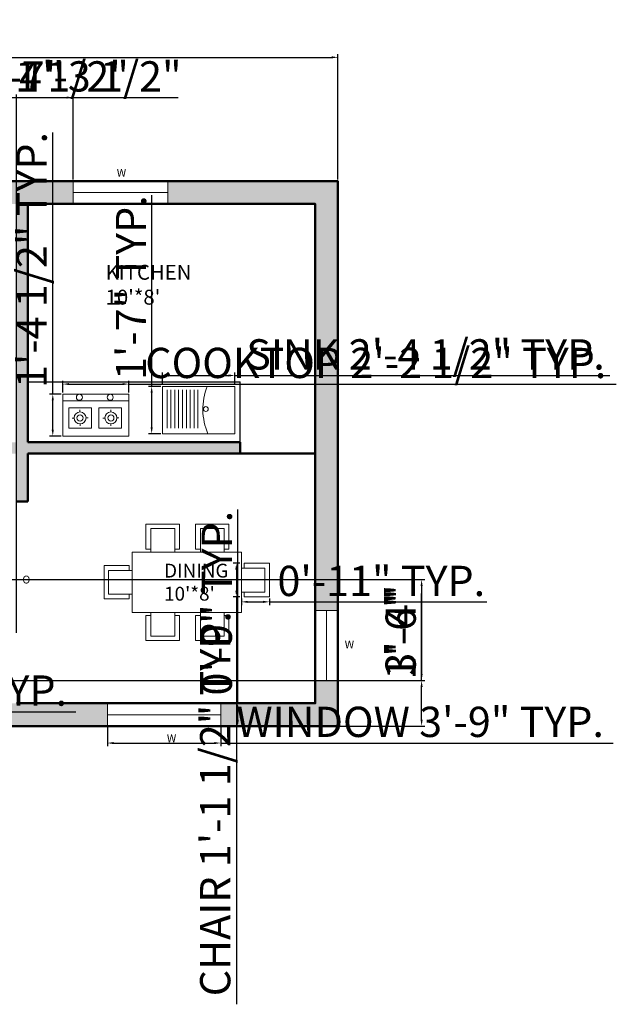
# Model space of a CAD drawing. Units: inches. Extents: x 2225 to 3094, y 1739 to 2599.
# Tile 5 of 5: x 2780 to 3017, y 2108 to 2498. Entities that reach past the tile are written whole.
import ezdxf

# ---------------------------------------------------------------- set-up
doc = ezdxf.new("R2010")
doc.units = ezdxf.units.IN
for name, color, linetype, lineweight in [('A-ANNO-DIMS', 2, 'Continuous', 18), ('A-ANNO-TEXT', 7, 'Continuous', 18), ('A-AREA-IDEN', 7, 'Continuous', 18), ('A-EQPM', 8, 'Continuous', 18), ('A-FLOR-CASE', 9, 'Continuous', 25), ('A-FLOR-FIXT', 9, 'Continuous', 18), ('A-FURN', 8, 'Continuous', 18), ('A-WALL-PATT', 160, 'Continuous', 13), ('WALL', 7, 'Continuous', 50), ('WINDOW', 130, 'Continuous', 18)]:
    doc.layers.add(name, color=color, linetype=linetype, lineweight=lineweight)
doc.styles.get("Standard").update_dxf_attribs({"font": 'arial.ttf'})
doc.dimstyles.new('ISO-25', dxfattribs={"dimtxt": 12, "dimasz": 2.5, "dimexe": 1.25, "dimexo": 0.625, "dimtad": 1, "dimdec": 0, "dimlunit": 4, "dimtxsty": 'Standard', "dimcen": 2.5, "dimadec": 0, "dimazin": 0, "dimtfac": 1, "dimtdec": 0, "dimtmove": 0, "dimatfit": 3, "dimfxl": 1, "dimarcsym": 0})

# ---------------------------------------------------------------- blocks, each defined once
blk = doc.blocks.new('*D5')
at = {"layer": 'A-ANNO-DIMS', "color": 0, "lineweight": -2, "transparency": 16777216}
for p, q in [((2282.56, 2434.95), (2282.56, 2484.67)), ((2285.06, 2483.42), (2904.06, 2483.42)), ((2906.56, 2434.95), (2906.56, 2484.67))]:
    blk.add_line(p, q, dxfattribs=at)
at = {"layer": 'A-ANNO-DIMS', "color": 0, "transparency": 16777216}
for points in [[(2285.06, 2483.83), (2285.06, 2483), (2282.56, 2483.42)], [(2904.06, 2483.83), (2904.06, 2483), (2906.56, 2483.42)]]:
    blk.add_solid(points, dxfattribs=at)
at = {"layer": 'Defpoints', "color": 0, "transparency": 16777216}
for p in [(2906.56, 2483.42), (2282.56, 2434.33), (2906.56, 2434.33)]:
    blk.add_point(p, dxfattribs=at)
at = {"layer": 'A-ANNO-DIMS', "color": 0, "transparency": 16777216, "insert": (2594.56, 2490.17), "char_height": 12, "attachment_point": 5}
blk.add_mtext("52'", dxfattribs=at)
blk = doc.blocks.new('CHAIR-DINING')
for p, q in [((0, 1.13), (0, 11.11)), ((0, 11.11), (13.29, 11.11)), ((13.29, 1.13), (13.29, 11.11)), ((1.95, 1.13), (0, 1.13)), ((13.29, 1.13), (11.43, 1.13))]:
    blk.add_line(p, q)
blk.add_lwpolyline([(1.95, 0), (11.43, 0), (11.43, 9.33), (1.95, 9.33)], close=True)
blk = doc.blocks.new('TABLE-DINING')
blk.add_lwpolyline([(0, 23.93), (43.3, 23.93), (43.3, 0), (0, 0)], close=True)
blk = doc.blocks.new('COOKTOP-TWO-BURNER')
for p, q in [((0, 13.93), (26.27, 13.93)), ((6.81, 9.56), (6.81, 10.38)), ((19.02, 9.56), (19.02, 10.38)), ((4.52, 7.14), (3.73, 7.14)), ((6.9, 4.82), (6.9, 4.11)), ((9.26, 7.23), (10.04, 7.23)), ((16.73, 7.14), (15.94, 7.14)), ((19.11, 4.82), (19.11, 4.11)), ((21.47, 7.23), (22.24, 7.23))]:
    blk.add_line(p, q)
for points in [[(0, 0), (26.27, 0), (26.27, 16.66), (0, 16.66)], [(2.47, 11.19), (11.48, 11.19), (11.48, 3.09), (2.47, 3.09)], [(14.27, 11.19), (23.28, 11.19), (23.28, 3.09), (14.27, 3.09)]]:
    blk.add_lwpolyline(points, close=True)
for centre, radius in [((6.64, 15.37), 1.2), ((18.83, 15.37), 1.2), ((6.89, 7.19), 2.37), ((6.89, 7.19), 1.23), ((19.1, 7.19), 2.37), ((19.1, 7.19), 1.23)]:
    blk.add_circle(centre, radius)
blk = doc.blocks.new('SINK-DRAINBOARD')
for p, q in [((1.79, 17.4), (1.79, 2.15)), ((3.32, 17.4), (3.32, 2.15)), ((4.85, 17.4), (4.85, 2.15)), ((6.38, 17.4), (6.38, 2.15)), ((7.91, 17.4), (7.91, 2.15)), ((9.44, 17.4), (9.44, 2.15)), ((10.98, 17.4), (10.98, 2.15)), ((12.51, 17.4), (12.51, 2.15)), ((14.04, 17.4), (14.04, 2.15))]:
    blk.add_line(p, q)
blk.add_lwpolyline([(0, 0), (28.72, 0), (28.72, 18.77), (0, 18.77)], close=True)
blk.add_circle((17.16, 9.78), 0.951)
blk.add_arc((40.38, 9.7), 24.39, 158.1829, 203.4296)
blk = doc.blocks.new('WIN-37P6IN')
blk.add_line((0, 4.5), (37.6, 4.5))
blk.add_lwpolyline([(37.6, 0), (0, 0), (0, 9), (37.6, 9)], close=True)
blk = doc.blocks.new('WIN-44P9IN')
blk.add_line((0, 4.5), (44.94, 4.5))
blk.add_lwpolyline([(0, 0), (44.94, 0), (44.94, 9), (0, 9)], close=True)
blk = doc.blocks.new('WIN-27P8IN')
blk.add_line((4.5, 0), (4.5, 27.82))
blk.add_lwpolyline([(0, 0), (9, 0), (9, 27.82), (0, 27.82)], close=True)
blk = doc.blocks.new('KITCHEN-COUNTER-RUN')
for p, q in [((0, 0), (0, 24)), ((0, 24), (84.25, 24)), ((84.25, 0), (84.25, 24))]:
    blk.add_line(p, q)
blk = doc.blocks.new('*D28')
at = {"layer": 'A-ANNO-DIMS', "color": 0, "lineweight": -2, "transparency": 16777216}
for p, q in [((2867.63, 2282.83), (2865.01, 2282.83)), ((2866.26, 2280.33), (2866.26, 2272.05)), ((2867.63, 2269.55), (2865.01, 2269.55)), ((2866.26, 2269.55), (2866.26, 2108.01))]:
    blk.add_line(p, q, dxfattribs=at)
at = {"layer": 'A-ANNO-DIMS', "color": 0, "transparency": 16777216}
for points in [[(2865.84, 2280.33), (2866.68, 2280.33), (2866.26, 2282.83)], [(2865.84, 2272.05), (2866.68, 2272.05), (2866.26, 2269.55)]]:
    blk.add_solid(points, dxfattribs=at)
at = {"layer": 'Defpoints', "color": 0, "transparency": 16777216}
for p in [(2868.25, 2282.83), (2866.26, 2269.55), (2868.25, 2269.55)]:
    blk.add_point(p, dxfattribs=at)
at = {"layer": 'A-ANNO-DIMS', "color": 0, "transparency": 16777216, "insert": (2859.43, 2187.53), "char_height": 12, "attachment_point": 5, "rotation": 90}
blk.add_mtext('CHAIR 1\'-1 1/2" TYP.', dxfattribs=at)
blk = doc.blocks.new('*D29')
at = {"layer": 'A-ANNO-DIMS', "color": 0, "lineweight": -2, "transparency": 16777216}
for p, q in [((2868.25, 2268.92), (2868.25, 2266.31)), ((2879.36, 2268.92), (2879.36, 2266.31)), ((2870.75, 2267.56), (2876.86, 2267.56)), ((2879.36, 2267.56), (2965.58, 2267.56))]:
    blk.add_line(p, q, dxfattribs=at)
at = {"layer": 'A-ANNO-DIMS', "color": 0, "transparency": 16777216}
for points in [[(2870.75, 2267.97), (2870.75, 2267.14), (2868.25, 2267.56)], [(2876.86, 2267.97), (2876.86, 2267.14), (2879.36, 2267.56)]]:
    blk.add_solid(points, dxfattribs=at)
at = {"layer": 'Defpoints', "color": 0, "transparency": 16777216}
for p in [(2868.25, 2269.55), (2879.36, 2269.55), (2879.36, 2267.56)]:
    blk.add_point(p, dxfattribs=at)
at = {"layer": 'A-ANNO-DIMS', "color": 0, "transparency": 16777216, "insert": (2923.72, 2274.31), "char_height": 12, "attachment_point": 5}
blk.add_mtext('0\'-11" TYP.', dxfattribs=at)
blk = doc.blocks.new('*D32')
at = {"layer": 'A-ANNO-DIMS', "color": 0, "lineweight": -2, "transparency": 16777216}
for p, q in [((2608.3, 2232.07), (2608.3, 2222.75)), ((2666.2, 2232.07), (2666.2, 2222.75)), ((2610.8, 2224), (2663.7, 2224)), ((2666.2, 2224), (2802.66, 2224))]:
    blk.add_line(p, q, dxfattribs=at)
at = {"layer": 'A-ANNO-DIMS', "color": 0, "transparency": 16777216}
for points in [[(2610.8, 2224.42), (2610.8, 2223.59), (2608.3, 2224)], [(2663.7, 2224.42), (2663.7, 2223.59), (2666.2, 2224)]]:
    blk.add_solid(points, dxfattribs=at)
at = {"layer": 'Defpoints', "color": 0, "transparency": 16777216}
for p in [(2608.3, 2232.69), (2666.2, 2232.69), (2666.2, 2224)]:
    blk.add_point(p, dxfattribs=at)
at = {"layer": 'A-ANNO-DIMS', "color": 0, "transparency": 16777216, "insert": (2735.68, 2230.84), "char_height": 12, "attachment_point": 5}
blk.add_mtext('SOFA 4\'-10" TYP.', dxfattribs=at)
blk = doc.blocks.new('*D38')
at = {"layer": 'A-ANNO-DIMS', "color": 0, "lineweight": -2, "transparency": 16777216}
for p, q in [((2797.42, 2350.57), (2797.42, 2355.14)), ((2799.92, 2353.89), (2821.19, 2353.89)), ((2823.69, 2350.57), (2823.69, 2355.14)), ((2823.69, 2353.89), (3016.9, 2353.89))]:
    blk.add_line(p, q, dxfattribs=at)
at = {"layer": 'A-ANNO-DIMS', "color": 0, "transparency": 16777216}
for points in [[(2799.92, 2354.3), (2799.92, 2353.47), (2797.42, 2353.89)], [(2821.19, 2354.3), (2821.19, 2353.47), (2823.69, 2353.89)]]:
    blk.add_solid(points, dxfattribs=at)
at = {"layer": 'Defpoints', "color": 0, "transparency": 16777216}
for p in [(2823.69, 2353.89), (2797.42, 2349.95), (2823.69, 2349.95)]:
    blk.add_point(p, dxfattribs=at)
at = {"layer": 'A-ANNO-DIMS', "color": 0, "transparency": 16777216, "insert": (2921.55, 2360.72), "char_height": 12, "attachment_point": 5}
blk.add_mtext('COOKTOP 2\'-2 1/2" TYP.', dxfattribs=at)
blk = doc.blocks.new('*D39')
at = {"layer": 'A-ANNO-DIMS', "color": 0, "lineweight": -2, "transparency": 16777216}
for p, q in [((2793.48, 2349.95), (2793.48, 2453.67)), ((2796.79, 2349.95), (2792.23, 2349.95)), ((2793.48, 2335.78), (2793.48, 2347.45)), ((2796.79, 2333.28), (2792.23, 2333.28))]:
    blk.add_line(p, q, dxfattribs=at)
at = {"layer": 'A-ANNO-DIMS', "color": 0, "transparency": 16777216}
for points in [[(2793.06, 2347.45), (2793.89, 2347.45), (2793.48, 2349.95)], [(2793.06, 2335.78), (2793.89, 2335.78), (2793.48, 2333.28)]]:
    blk.add_solid(points, dxfattribs=at)
at = {"layer": 'Defpoints', "color": 0, "transparency": 16777216}
for p in [(2793.48, 2349.95), (2797.42, 2349.95), (2797.42, 2333.28)]:
    blk.add_point(p, dxfattribs=at)
at = {"layer": 'A-ANNO-DIMS', "color": 0, "transparency": 16777216, "insert": (2786.65, 2403.06), "char_height": 12, "attachment_point": 5, "rotation": 90}
blk.add_mtext('1\'-4 1/2" TYP.', dxfattribs=at)
blk = doc.blocks.new('*D40')
at = {"layer": 'A-ANNO-DIMS', "color": 0, "lineweight": -2, "transparency": 16777216}
for p, q in [((2837, 2353.6), (2837, 2358.53)), ((2865.72, 2353.6), (2865.72, 2358.53)), ((2839.5, 2357.28), (2863.22, 2357.28)), ((2865.72, 2357.28), (3014.3, 2357.28))]:
    blk.add_line(p, q, dxfattribs=at)
at = {"layer": 'A-ANNO-DIMS', "color": 0, "transparency": 16777216}
for points in [[(2839.5, 2357.7), (2839.5, 2356.87), (2837, 2357.28)], [(2863.22, 2357.7), (2863.22, 2356.87), (2865.72, 2357.28)]]:
    blk.add_solid(points, dxfattribs=at)
at = {"layer": 'Defpoints', "color": 0, "transparency": 16777216}
for p in [(2865.72, 2357.28), (2837, 2352.98), (2865.72, 2352.98)]:
    blk.add_point(p, dxfattribs=at)
at = {"layer": 'A-ANNO-DIMS', "color": 0, "transparency": 16777216, "insert": (2941.26, 2364.11), "char_height": 12, "attachment_point": 5}
blk.add_mtext('SINK 2\'-4 1/2" TYP.', dxfattribs=at)
blk = doc.blocks.new('*D41')
at = {"layer": 'A-ANNO-DIMS', "color": 0, "lineweight": -2, "transparency": 16777216}
for p, q in [((2832.69, 2352.98), (2832.69, 2428.74)), ((2836.38, 2352.98), (2831.44, 2352.98)), ((2832.69, 2336.71), (2832.69, 2350.48)), ((2836.38, 2334.21), (2831.44, 2334.21))]:
    blk.add_line(p, q, dxfattribs=at)
at = {"layer": 'A-ANNO-DIMS', "color": 0, "transparency": 16777216}
for points in [[(2832.28, 2350.48), (2833.11, 2350.48), (2832.69, 2352.98)], [(2832.28, 2336.71), (2833.11, 2336.71), (2832.69, 2334.21)]]:
    blk.add_solid(points, dxfattribs=at)
at = {"layer": 'Defpoints', "color": 0, "transparency": 16777216}
for p in [(2832.69, 2352.98), (2837, 2352.98), (2837, 2334.21)]:
    blk.add_point(p, dxfattribs=at)
at = {"layer": 'A-ANNO-DIMS', "color": 0, "transparency": 16777216, "insert": (2826.04, 2392.11), "char_height": 12, "attachment_point": 5, "rotation": 90}
blk.add_mtext('1\'-7" TYP.', dxfattribs=at)
blk = doc.blocks.new('*D48')
at = {"layer": 'A-ANNO-DIMS', "color": 0, "lineweight": -2, "transparency": 16777216}
for p, q in [((2815.14, 2217.7), (2815.14, 2210.34)), ((2860.08, 2217.7), (2860.08, 2210.34)), ((2817.64, 2211.59), (2857.58, 2211.59)), ((2860.08, 2211.59), (3015.68, 2211.59))]:
    blk.add_line(p, q, dxfattribs=at)
at = {"layer": 'A-ANNO-DIMS', "color": 0, "transparency": 16777216}
for points in [[(2817.64, 2212), (2817.64, 2211.17), (2815.14, 2211.59)], [(2857.58, 2212), (2857.58, 2211.17), (2860.08, 2211.59)]]:
    blk.add_solid(points, dxfattribs=at)
at = {"layer": 'Defpoints', "color": 0, "transparency": 16777216}
for p in [(2815.14, 2218.33), (2860.08, 2218.33), (2860.08, 2211.59)]:
    blk.add_point(p, dxfattribs=at)
at = {"layer": 'A-ANNO-DIMS', "color": 0, "transparency": 16777216, "insert": (2939.13, 2218.43), "char_height": 12, "attachment_point": 5}
blk.add_mtext('WINDOW 3\'-9" TYP.', dxfattribs=at)
blk = doc.blocks.new('*D49')
at = {"layer": 'A-ANNO-DIMS', "color": 0, "lineweight": -2, "transparency": 16777216}
for p, q in [((2866.82, 2227.33), (2866.82, 2304.22)), ((2860.7, 2227.33), (2868.07, 2227.33)), ((2866.82, 2220.83), (2866.82, 2224.83)), ((2860.7, 2218.33), (2868.07, 2218.33))]:
    blk.add_line(p, q, dxfattribs=at)
at = {"layer": 'A-ANNO-DIMS', "color": 0, "transparency": 16777216}
for points in [[(2866.4, 2224.83), (2867.23, 2224.83), (2866.82, 2227.33)], [(2866.4, 2220.83), (2867.23, 2220.83), (2866.82, 2218.33)]]:
    blk.add_solid(points, dxfattribs=at)
at = {"layer": 'Defpoints', "color": 0, "transparency": 16777216}
for p in [(2860.08, 2227.33), (2866.82, 2227.33), (2860.08, 2218.33)]:
    blk.add_point(p, dxfattribs=at)
at = {"layer": 'A-ANNO-DIMS', "color": 0, "transparency": 16777216, "insert": (2860.06, 2267.03), "char_height": 12, "attachment_point": 5, "rotation": 90}
blk.add_mtext('0\'-9" TYP.', dxfattribs=at)
blk = doc.blocks.new('*D61')
at = {"layer": 'A-ANNO-DIMS', "color": 0, "lineweight": -2, "transparency": 16777216}
for p, q in [((2720.79, 2434.95), (2720.79, 2468.73)), ((2723.29, 2467.48), (2755.89, 2467.48)), ((2758.39, 2434.95), (2758.39, 2468.73)), ((2758.39, 2467.48), (2821.99, 2467.48))]:
    blk.add_line(p, q, dxfattribs=at)
at = {"layer": 'A-ANNO-DIMS', "color": 0, "transparency": 16777216}
for points in [[(2723.29, 2467.89), (2723.29, 2467.06), (2720.79, 2467.48)], [(2755.89, 2467.89), (2755.89, 2467.06), (2758.39, 2467.48)]]:
    blk.add_solid(points, dxfattribs=at)
at = {"layer": 'Defpoints', "color": 0, "transparency": 16777216}
for p in [(2758.39, 2467.48), (2720.79, 2434.33), (2758.39, 2434.33)]:
    blk.add_point(p, dxfattribs=at)
at = {"layer": 'A-ANNO-DIMS', "color": 0, "transparency": 16777216, "insert": (2791.44, 2474.31), "char_height": 12, "attachment_point": 5}
blk.add_mtext('3\'-1 1/2"', dxfattribs=at)
blk = doc.blocks.new('*D62')
at = {"layer": 'A-ANNO-DIMS', "color": 0, "lineweight": -2, "transparency": 16777216}
for p, q in [((2758.39, 2434.95), (2758.39, 2468.73)), ((2760.89, 2467.48), (2799.04, 2467.48)), ((2801.54, 2434.95), (2801.54, 2468.73))]:
    blk.add_line(p, q, dxfattribs=at)
at = {"layer": 'A-ANNO-DIMS', "color": 0, "transparency": 16777216}
for points in [[(2760.89, 2467.89), (2760.89, 2467.06), (2758.39, 2467.48)], [(2799.04, 2467.89), (2799.04, 2467.06), (2801.54, 2467.48)]]:
    blk.add_solid(points, dxfattribs=at)
at = {"layer": 'Defpoints', "color": 0, "transparency": 16777216}
for p in [(2801.54, 2467.48), (2758.39, 2434.33), (2801.54, 2434.33)]:
    blk.add_point(p, dxfattribs=at)
at = {"layer": 'A-ANNO-DIMS', "color": 0, "transparency": 16777216, "insert": (2779.97, 2474.23), "char_height": 12, "attachment_point": 5}
blk.add_mtext('3\'-7"', dxfattribs=at)
blk = doc.blocks.new('*D65')
at = {"layer": 'A-ANNO-DIMS', "color": 0, "lineweight": -2, "transparency": 16777216}
for p, q in [((2939.71, 2236.32), (2939.71, 2270.83)), ((2907.18, 2236.32), (2940.96, 2236.32)), ((2939.71, 2220.83), (2939.71, 2233.82)), ((2907.18, 2218.33), (2940.96, 2218.33))]:
    blk.add_line(p, q, dxfattribs=at)
at = {"layer": 'A-ANNO-DIMS', "color": 0, "transparency": 16777216}
for points in [[(2939.29, 2233.82), (2940.12, 2233.82), (2939.71, 2236.32)], [(2939.29, 2220.83), (2940.12, 2220.83), (2939.71, 2218.33)]]:
    blk.add_solid(points, dxfattribs=at)
at = {"layer": 'Defpoints', "color": 0, "transparency": 16777216}
for p in [(2906.56, 2236.32), (2939.71, 2236.32), (2906.56, 2218.33)]:
    blk.add_point(p, dxfattribs=at)
at = {"layer": 'A-ANNO-DIMS', "color": 0, "transparency": 16777216, "insert": (2932.96, 2254.82), "char_height": 12, "attachment_point": 5, "rotation": 90}
blk.add_mtext('1\'-6"', dxfattribs=at)
blk = doc.blocks.new('*D68')
at = {"layer": 'A-ANNO-DIMS', "color": 0, "lineweight": -2, "transparency": 16777216}
for p, q in [((2500.68, 2276.4), (2940.96, 2276.4)), ((2939.71, 2273.9), (2939.71, 2238.9)), ((2500.68, 2236.4), (2940.96, 2236.4))]:
    blk.add_line(p, q, dxfattribs=at)
at = {"layer": 'A-ANNO-DIMS', "color": 0, "transparency": 16777216}
for points in [[(2939.29, 2273.9), (2940.12, 2273.9), (2939.71, 2276.4)], [(2939.29, 2238.9), (2940.12, 2238.9), (2939.71, 2236.4)]]:
    blk.add_solid(points, dxfattribs=at)
at = {"layer": 'Defpoints', "color": 0, "transparency": 16777216}
for p in [(2500.06, 2276.4), (2500.06, 2236.4), (2939.71, 2236.4)]:
    blk.add_point(p, dxfattribs=at)
at = {"layer": 'A-ANNO-DIMS', "color": 0, "transparency": 16777216, "insert": (2932.95, 2256.4), "char_height": 12, "attachment_point": 5, "rotation": 90}
blk.add_mtext('3\'-4"', dxfattribs=at)
blk = doc.blocks.new('*D74')
at = {"layer": 'A-ANNO-DIMS', "color": 0, "lineweight": -2, "transparency": 16777216}
for p, q in [((2727.64, 2255.24), (2727.64, 2468.73)), ((2730.14, 2467.48), (2776.56, 2467.48)), ((2779.06, 2255.24), (2779.06, 2468.73)), ((2779.06, 2467.48), (2843.15, 2467.48))]:
    blk.add_line(p, q, dxfattribs=at)
at = {"layer": 'A-ANNO-DIMS', "color": 0, "transparency": 16777216}
for points in [[(2730.14, 2467.89), (2730.14, 2467.06), (2727.64, 2467.48)], [(2776.56, 2467.89), (2776.56, 2467.06), (2779.06, 2467.48)]]:
    blk.add_solid(points, dxfattribs=at)
at = {"layer": 'Defpoints', "color": 0, "transparency": 16777216}
for p in [(2779.06, 2467.48), (2727.64, 2254.61), (2779.06, 2254.61)]:
    blk.add_point(p, dxfattribs=at)
at = {"layer": 'A-ANNO-DIMS', "color": 0, "transparency": 16777216, "insert": (2812.35, 2474.31), "char_height": 12, "attachment_point": 5}
blk.add_mtext('4\'-3 1/2"', dxfattribs=at)

msp = doc.modelspace()

# ---------------------------------------------------------------- hatches: boundary and pattern name
at = {"layer": 'A-WALL-PATT'}
h = msp.add_hatch(color=256, dxfattribs=at)
h.dxf.hatch_style = 1
h.paths.add_polyline_path([(2445.16, 2434.33), (2282.56, 2434.33), (2282.56, 2366.97), (2291.56, 2366.97), (2291.56, 2425.33), (2445.16, 2425.33)], flags=17)
h.paths.add_polyline_path([(2528.69, 2434.33), (2482.76, 2434.33), (2482.76, 2425.33), (2495.56, 2425.33), (2495.56, 2414.78), (2499.34, 2414.78, -0.007163), (2500.06, 2414.76), (2500.06, 2425.33), (2528.69, 2425.33)], flags=17)
h.paths.add_polyline_path([(2867.81, 2330.83), (2783.56, 2330.83), (2783.56, 2354.83), (2783.56, 2425.33), (2801.54, 2425.33), (2801.54, 2434.33), (2758.39, 2434.33), (2758.39, 2425.33), (2779.06, 2425.33), (2779.06, 2330.83), (2767.43, 2330.83), (2767.43, 2326.33), (2779.06, 2326.33), (2779.06, 2307.37), (2783.56, 2307.37), (2783.56, 2326.33), (2867.81, 2326.33)])
h.paths.add_polyline_path([(2906.56, 2434.33), (2839.14, 2434.33), (2839.14, 2425.33), (2897.56, 2425.33), (2897.56, 2330.83), (2897.56, 2326.33), (2897.56, 2264.13), (2906.56, 2264.13)])
h.paths.add_polyline_path([(2906.56, 2236.32), (2897.56, 2236.32), (2897.56, 2227.33), (2860.08, 2227.33), (2860.08, 2218.33), (2906.56, 2218.33)])
h.paths.add_polyline_path([(2815.14, 2227.33), (2783.56, 2227.33), (2779.06, 2227.33), (2727.64, 2227.33), (2606.48, 2227.33), (2606.48, 2218.33), (2815.14, 2218.33)])
h.paths.add_polyline_path([(2780.45, 2273.09), (2785.35, 2273.09), (2785.35, 2279.46), (2780.45, 2279.46)], flags=9)
h.paths.add_polyline_path([(2500.16, 2250.57), (2508.42, 2250.57), (2508.42, 2256.93), (2500.16, 2256.93)], flags=25)
h.paths.add_polyline_path([(2745.49, 2326.59), (2750.15, 2326.59), (2750.15, 2332.96), (2745.49, 2332.96)], flags=9)
h.paths.add_polyline_path([(2651.86, 2391.09), (2656.53, 2391.09), (2656.53, 2397.46), (2651.86, 2397.46)], flags=9)
h.paths.add_polyline_path([(2493.47, 2330.16), (2498.13, 2330.16), (2498.13, 2336.53), (2493.47, 2336.53)], flags=25)
h.paths.add_polyline_path([(2530.27, 2348.62), (2534.93, 2348.62), (2534.93, 2354.99), (2530.27, 2354.99)], flags=25)
h.paths.add_polyline_path([(2432.89, 2282.56), (2450.26, 2282.56), (2450.26, 2294.09), (2432.89, 2294.09)], flags=25)
h.paths.add_polyline_path([(2735.79, 2240.68), (2748.37, 2240.68), (2748.37, 2247.05), (2735.79, 2247.05)], flags=9)
h.paths.add_polyline_path([(2717.02, 2288.94), (2747.35, 2288.94), (2747.35, 2300.47), (2717.02, 2300.47)], flags=9)
h.paths.add_polyline_path([(2839.5, 2270.61), (2856.29, 2270.61), (2856.29, 2282.14), (2839.5, 2282.14)], flags=25)
h.paths.add_polyline_path([(2825.64, 2385.51), (2846.28, 2385.51), (2846.28, 2397.04), (2825.64, 2397.04)], flags=25)
h.paths.add_polyline_path([(2692.05, 2396.34), (2722.05, 2396.34), (2722.05, 2407.87), (2692.05, 2407.87)], flags=9)
h.paths.add_polyline_path([(2282.56, 2366.97), (2291.56, 2366.97), (2291.56, 2425.33), (2445.16, 2425.33), (2445.16, 2434.33), (2282.56, 2434.33)])
h.paths.add_polyline_path([(2291.56, 2341.62), (2282.56, 2341.62), (2282.56, 2218.33), (2550.8, 2218.33), (2550.8, 2227.33), (2500.06, 2227.33), (2500.06, 2236.4), (2495.56, 2236.4), (2495.56, 2227.33), (2291.56, 2227.33), (2291.56, 2306.83), (2327.56, 2306.83), (2495.56, 2306.83), (2495.56, 2276.4), (2500.06, 2276.4), (2500.06, 2306.83), (2500.06, 2317.06), (2495.56, 2317.06), (2495.56, 2311.33), (2291.56, 2311.33)])

# ---------------------------------------------------------------- linework, layer by layer
at = {"layer": 'WALL'}
for p, q in [((2783.56, 2425.33), (2783.56, 2330.83)), ((2897.56, 2326.33), (2897.56, 2334.34)), ((2783.56, 2330.83), (2867.81, 2330.83)), ((2867.81, 2326.33), (2867.81, 2330.83)), ((2783.56, 2326.33), (2783.56, 2307.37)), ((2783.56, 2326.33), (2897.56, 2326.33)), ((2779.06, 2307.37), (2783.56, 2307.37)), ((2779.06, 2227.33), (2783.56, 2227.33)), ((2897.56, 2227.33), (2783.56, 2227.33))]:
    msp.add_line(p, q, dxfattribs=at)
msp.add_lwpolyline([(2282.56, 2218.33), (2906.56, 2218.33), (2906.56, 2434.33), (2282.56, 2434.33)], close=True, dxfattribs=at)
for points in [[(2897.56, 2330.83), (2897.56, 2425.33), (2783.56, 2425.33)], [(2783.56, 2227.33), (2897.56, 2227.33), (2897.56, 2326.33)]]:
    msp.add_lwpolyline(points, dxfattribs=at)

# ---------------------------------------------------------------- block references
at = {"layer": 'A-EQPM'}
msp.add_blockref('COOKTOP-TWO-BURNER', (2797.42, 2333.28), dxfattribs=at)
at = {"layer": 'A-FLOR-CASE'}
msp.add_blockref('KITCHEN-COUNTER-RUN', (2783.56, 2330.83), dxfattribs=at)
at = {"layer": 'A-FLOR-FIXT'}
msp.add_blockref('SINK-DRAINBOARD', (2837, 2334.21), dxfattribs=at)
at = {"layer": 'A-FURN'}
for name, p in [('CHAIR-DINING', (2830.39, 2287.27)), ('CHAIR-DINING', (2850.04, 2287.27)), ('TABLE-DINING', (2824.95, 2263.34))]:
    msp.add_blockref(name, p, dxfattribs=at)
at = {"layer": 'A-FURN', "extrusion": (0, 0, -1), "zscale": -1}
for p, rotation in [((-2824.95, 2281.99), 269.9999999999983), ((-2830.39, 2263.34), 180), ((-2850.04, 2263.34), 180)]:
    msp.add_blockref('CHAIR-DINING', p, dxfattribs=dict(at, rotation=rotation))
at = {"layer": 'A-FURN', "rotation": 269.9999999999885}
msp.add_blockref('CHAIR-DINING', (2868.25, 2282.83), dxfattribs=at)
at = {"layer": 'WINDOW'}
for name, p in [('WIN-37P6IN', (2801.54, 2425.33)), ('WIN-27P8IN', (2897.56, 2236.32)), ('WIN-44P9IN', (2815.14, 2218.33))]:
    msp.add_blockref(name, p, dxfattribs=at)

# ---------------------------------------------------------------- texts
at = {"layer": 'A-ANNO-TEXT', "char_height": 3.09, "attachment_point": 1}
for s, insert in [('W', (2818.86, 2439.18)), ('\\pxt3;O', (2781.43, 2277.93)), ('W', (2909.23, 2252.2)), ('W', (2838.73, 2215))]:
    msp.add_mtext_dynamic_manual_height_columns(s, width=49.525, gutter_width=15.45, heights=[0], dxfattribs=dict(at, insert=insert))
at = {"layer": 'A-AREA-IDEN', "attachment_point": 1}
for s, width, gutter_width, heights, insert, char_height in [("KITCHEN\\P10'*8'", 94.8443, 29.59, [0], (2814.43, 2401.16), 5.917), ("DINING\\P10'*8'", 87.8531, 27.41, [14.83], (2837.63, 2282.67), 5.481)]:
    msp.add_mtext_dynamic_manual_height_columns(s, width=width, gutter_width=gutter_width, heights=heights, dxfattribs=dict(at, insert=insert, char_height=char_height))

# ---------------------------------------------------------------- dimensions: what is measured, and where the dimension line sits
at = {"layer": 'A-ANNO-DIMS'}
for base, p1, p2, override, picture, middle in [((2906.56, 2483.42), (2282.56, 2434.33), (2906.56, 2434.33), {"dimclrd": 0, "dimclre": 0, "dimclrt": 0}, '*D5', (2594.56, 2490.17)), ((2758.39, 2467.48), (2720.79, 2434.33), (2758.39, 2434.33), {"dimdec": 1, "dimlfac": 1, "dimrnd": 0, "dimzin": 1, "dimdsep": 46, "dimlunit": 4, "dimfrac": 2}, '*D61', (2791.44, 2474.31)), ((2779.06, 2467.48), (2727.64, 2254.61), (2779.06, 2254.61), {"dimdec": 1, "dimlfac": 1, "dimrnd": 0, "dimzin": 1, "dimdsep": 46, "dimlunit": 4, "dimfrac": 2}, '*D74', (2812.35, 2474.31)), ((2801.5388, 2467.4778), (2758.3918, 2434.3278), (2801.5388, 2434.3278), {"dimdec": 1, "dimlfac": 1, "dimrnd": 0, "dimzin": 1, "dimdsep": 46, "dimlunit": 4, "dimfrac": 2}, '*D62', (2779.9653, 2474.2337))]:
    dim = msp.add_linear_dim(base=base, p1=p1, p2=p2, dimstyle='ISO-25', override=override, dxfattribs=at)
    dim.commit()
    dim.dimension.update_dxf_attribs({"geometry": picture, "text_midpoint": middle})
for base, p1, p2, angle, text, picture, middle in [((2793.48, 2349.95), (2797.42, 2333.28), (2797.42, 2349.95), 90, '<> TYP.', '*D39', (2786.65, 2403.06)), ((2832.69, 2352.98), (2837, 2334.21), (2837, 2352.98), 90, '<> TYP.', '*D41', (2826.04, 2392.11)), ((2866.82, 2227.33), (2860.08, 2218.33), (2860.08, 2227.33), 90, '<> TYP.', '*D49', (2860.06, 2267.03)), ((2866.26, 2269.55), (2868.25, 2282.83), (2868.25, 2269.55), 270, 'CHAIR <> TYP.', '*D28', (2859.43, 2187.53))]:
    dim = msp.add_linear_dim(base=base, p1=p1, p2=p2, angle=angle, text=text, dimstyle='ISO-25', override={"dimdec": 1, "dimlfac": 1, "dimrnd": 0, "dimzin": 1, "dimdsep": 46, "dimlunit": 4, "dimfrac": 2}, dxfattribs=at)
    dim.commit()
    dim.dimension.update_dxf_attribs({"geometry": picture, "text_midpoint": middle})
for base, p1, p2, text, picture, middle in [((2865.72, 2357.28), (2837, 2352.98), (2865.72, 2352.98), 'SINK <> TYP.', '*D40', (2941.26, 2364.11)), ((2823.69, 2353.89), (2797.42, 2349.95), (2823.69, 2349.95), 'COOKTOP <> TYP.', '*D38', (2921.55, 2360.72)), ((2879.36, 2267.56), (2868.25, 2269.55), (2879.36, 2269.55), '<> TYP.', '*D29', (2923.72, 2274.31)), ((2666.2, 2224), (2608.3, 2232.69), (2666.2, 2232.69), 'SOFA <> TYP.', '*D32', (2735.68, 2230.84)), ((2860.08, 2211.59), (2815.14, 2218.33), (2860.08, 2218.33), 'WINDOW <> TYP.', '*D48', (2939.13, 2218.43))]:
    dim = msp.add_linear_dim(base=base, p1=p1, p2=p2, text=text, dimstyle='ISO-25', override={"dimdec": 1, "dimlfac": 1, "dimrnd": 0, "dimzin": 1, "dimdsep": 46, "dimlunit": 4, "dimfrac": 2}, dxfattribs=at)
    dim.commit()
    dim.dimension.update_dxf_attribs({"geometry": picture, "text_midpoint": middle})
for base, p1, p2, picture, middle in [((2939.71, 2236.4), (2500.06, 2276.4), (2500.06, 2236.4), '*D68', (2932.95, 2256.4)), ((2939.71, 2236.32), (2906.56, 2218.33), (2906.56, 2236.32), '*D65', (2932.96, 2254.82))]:
    dim = msp.add_linear_dim(base=base, p1=p1, p2=p2, angle=90, dimstyle='ISO-25', override={"dimdec": 1, "dimlfac": 1, "dimrnd": 0, "dimzin": 1, "dimdsep": 46, "dimlunit": 4, "dimfrac": 2}, dxfattribs=at)
    dim.commit()
    dim.dimension.update_dxf_attribs({"geometry": picture, "text_midpoint": middle})

doc.saveas('drawing.dxf')
